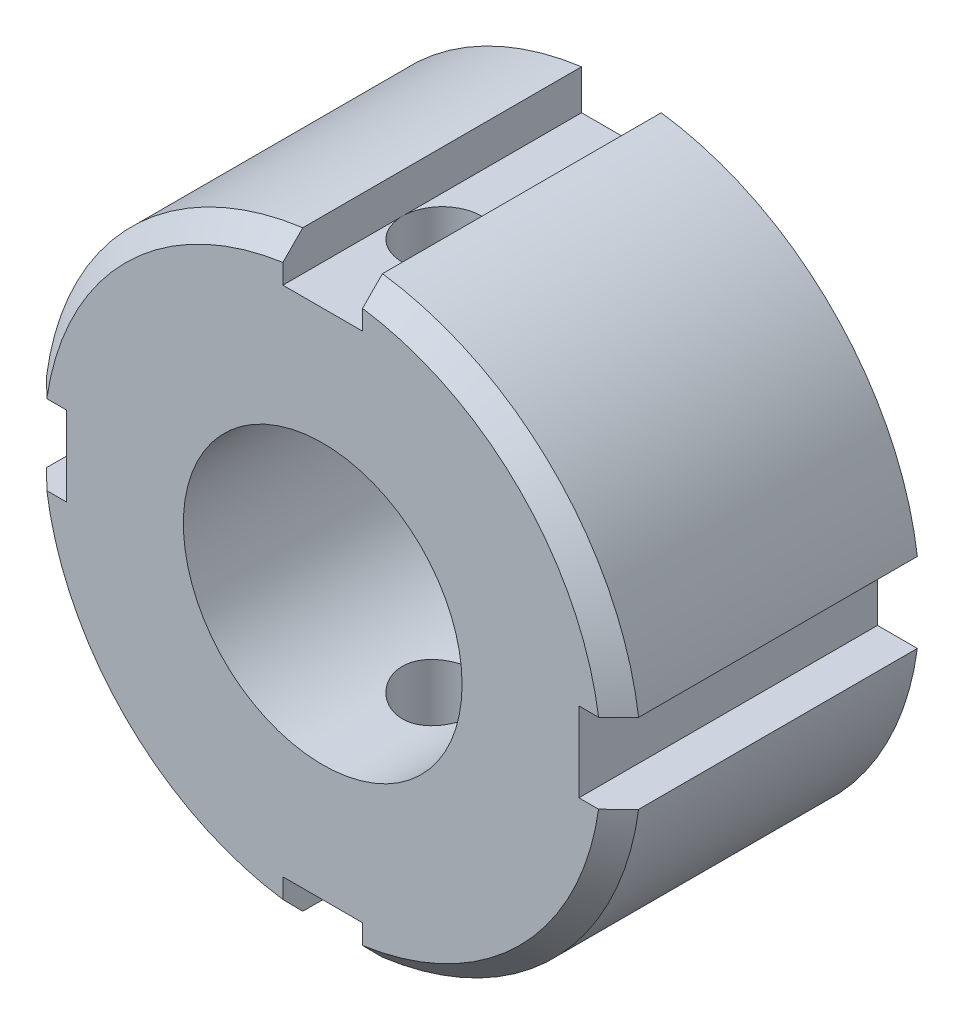
SolidWorks part; units mm, degrees
material "Plain Carbon Steel"
ref_plane "Front Plane" through (0, 0, 0) normal (0, 0, 1) x (1, 0, 0)
ref_plane "Top Plane" through (0, 0, 0) normal (0, 1, 0) x (1, 0, 0)
ref_plane "Right Plane" through (0, 0, 0) normal (1, 0, 0) x (0, 0, -1)
sketch "Slotted Nut Profile Ø30" plane through (0, 0, 0) normal (0, 0, 1) x (1, 0, 0)
  line L0 (0, -20.2412) -> (0, 21.4741) construction
  line L1 (2, 12.8661) -> (2, 14.8661)
  line L2 (-2, 12.8661) -> (-2, 14.8661)
  line L3 (-2, 12.8661) -> (2, 12.8661)
  line L4 (12.8661, 2) -> (14.8661, 2)
  line L5 (-2, -20.2412) -> (-2, 21.4741) construction
  line L6 (2, -20.2412) -> (2, 21.4741) construction
  line L7 (12.8661, 2) -> (12.8661, -2)
  line L8 (12.8661, -2) -> (14.8661, -2)
  line L9 (2, -12.8661) -> (2, -14.8661)
  line L10 (2, -12.8661) -> (-2, -12.8661)
  line L11 (-2, -12.8661) -> (-2, -14.8661)
  line L12 (-12.8661, -2) -> (-14.8661, -2)
  line L13 (-12.8661, -2) -> (-12.8661, 2)
  line L14 (-12.8661, 2) -> (-14.8661, 2)
  arc A0 (-2, 14.8661) -> (-14.8661, 2) centre (0, 0) ccw
  arc A1 (-14.8661, -2) -> (-2, -14.8661) centre (0, 0) ccw
  arc A2 (2, -14.8661) -> (14.8661, -2) centre (0, 0) ccw
  arc A3 (14.8661, 2) -> (2, 14.8661) centre (0, 0) ccw
  point P27 (0, 0)
  dimension "D1" = 30
  dimension "D4" = 2
  dimension "D2" = 2
  dimension "D3" = 2
  dimension "D5" = 4
extrude "Nut Body 15mm" add sketch "Slotted Nut Profile Ø30" along normal mid plane 15
hole_wizard "M16 Tapped Through Hole" positions "Sketch2" profile "Sketch3" tap size "M16" standard "DIN" end condition through all
sketch "Sketch2" plane through (0, 0, 7.5) normal (0, 0, 1) x (1, 0, 0)
  point P0 (0, 0)
sketch "Sketch3" plane through (0, 0, 7.5) normal (1, 0, 0) x (0, -1, 0)
  line L0 (0, 0) -> (0, 15)
  line L1 (0, 15) -> (7, 15)
  line L2 (7, 15) -> (7, 0)
  line L5 (7, 0) -> (0, 0)
  line L11 (0, -6.35) -> (0, 107.95) construction
  dimension "Thru Tap Drill Dia." = 14
  dimension "Thru Tap Drill Depth" = 15
cosmetic thread "Hole Thread1" parameters "D2"=16
chamfer "Edge Chamfer 1x45°" distance 1 angle 45 4 edges at (-10.6066, -10.6066, 7.5) (10.6066, -10.6066, 7.5) (10.6066, 10.6066, 7.5) (-10.6066, 10.6066, 7.5)
sketch "Cross Hole Ø4 Sketch" plane through (0, 0, 0) normal (0, 1, 0) x (1, 0, 0)
  line L0 (0, 7.5) -> (0, -7.5) construction
  line L1 (2, -7.5) -> (-2, -7.5) construction
  circle A0 centre (0, -1.5) radius 2
  dimension "D1" = 4
  dimension "D2" = 6
extrude "Cross Hole Ø4" cut sketch "Cross Hole Ø4 Sketch" against normal through all both and the other way through all
